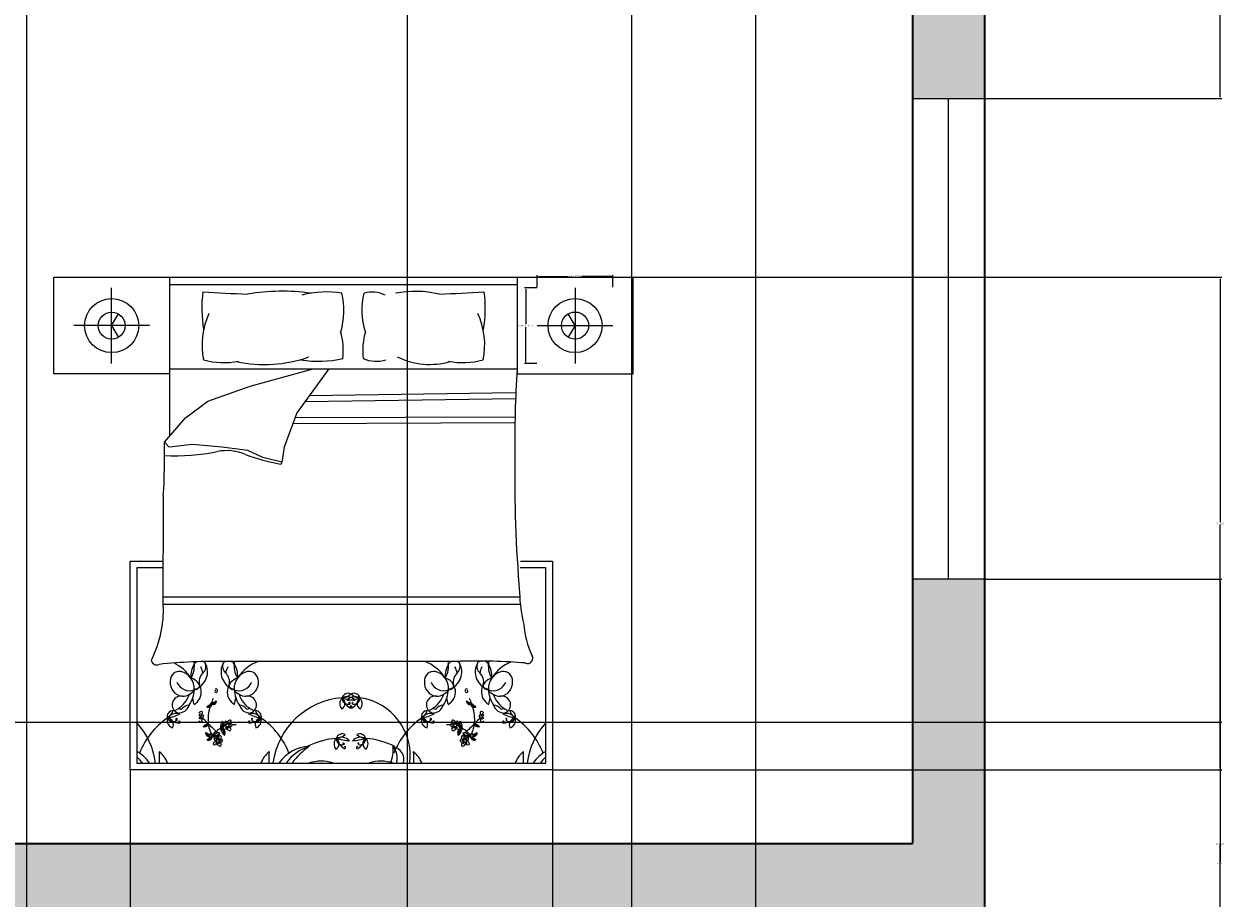
# Model space of a CAD drawing. Units: inches. Extents: x 0 to 423, y -517 to 94.
# Tile 5 of 8: x 273 to 423, y -270 to -160. Entities that reach past the tile are written whole.
import ezdxf

# ---------------------------------------------------------------- set-up
doc = ezdxf.new("R2010")
doc.units = ezdxf.units.IN
doc.header["$MEASUREMENT"] = 0
for name, color, linetype, lineweight in [('A-ANNO-DIMS', 2, 'Continuous', 18), ('A-FURN', 8, 'Continuous', 13), ('A-GLAZ', 4, 'Continuous', 18), ('A-WALL', 7, 'Continuous', 35)]:
    doc.layers.add(name, color=color, linetype=linetype, lineweight=lineweight)
doc.layers.add('A-WALL-PATT', color=30, linetype='Continuous', lineweight=13, true_color=0xf26722)
doc.styles.get("Standard").update_dxf_attribs({"font": 'arial.ttf'})
doc.dimstyles.get("Standard").update_dxf_attribs({"dimtxt": 0.18, "dimasz": 0.18, "dimexe": 0.18, "dimexo": 0.0625, "dimgap": 0.09, "dimtad": 0, "dimtih": 1, "dimtoh": 1, "dimdec": 0, "dimzin": 0, "dimdsep": 46, "dimlunit": 3, "dimtxsty": 'Standard', "dimcen": 0.09, "dimadec": 0, "dimazin": 0, "dimtfac": 1, "dimtdec": 0, "dimtofl": 0, "dimtmove": 0, "dimatfit": 3, "dimfxl": 1, "dimtolj": 1, "dimtzin": 0, "dimarcsym": 0})

# ---------------------------------------------------------------- blocks, each defined once
blk = doc.blocks.new('WIN-GLAZ-60IN')
for p, q in [((0, 60), (0, 0)), ((4.5, 60), (4.5, 0)), ((9, 0), (9, 60))]:
    blk.add_line(p, q)
blk = doc.blocks.new('BEDSIDE-LAMP-MEDIUM')
for p, q in [((4.72, 0), (4.72, 9.44)), ((9.44, 4.72), (0, 4.72))]:
    blk.add_line(p, q)
for points in [[(4.72, 4.72), (5.56, 6.18)], [(4.72, 4.72), (5.56, 3.26)]]:
    blk.add_lwpolyline(points)
for radius in [3.37, 1.69]:
    blk.add_circle((4.72, 4.72), radius)
blk = doc.blocks.new('*D26')
at = {"layer": 'A-ANNO-DIMS', "color": 0, "lineweight": -2, "transparency": 16777216}
for p, q in [((336.85, -193.39), (335.32, -193.39)), ((335.5, -193.57), (335.5, -197.93)), ((335.5, -202.66), (335.5, -198.3)), ((336.85, -202.84), (335.32, -202.84))]:
    blk.add_line(p, q, dxfattribs=at)
at = {"layer": 'A-ANNO-DIMS', "color": 0, "transparency": 16777216}
for points in [[(335.47, -193.57), (335.53, -193.57), (335.5, -193.39)], [(335.47, -202.66), (335.53, -202.66), (335.5, -202.84)]]:
    blk.add_solid(points, dxfattribs=at)
at = {"layer": 'Defpoints', "color": 0, "transparency": 16777216}
for p in [(336.91, -193.39), (335.5, -202.84), (336.91, -202.84)]:
    blk.add_point(p, dxfattribs=at)
at = {"layer": 'A-ANNO-DIMS', "color": 0, "transparency": 16777216, "insert": (335.5, -198.12), "char_height": 0.18, "attachment_point": 5}
blk.add_mtext('\\A1;LAMP 0\'-9 1/2" TYP.', dxfattribs=at)
blk = doc.blocks.new('*D27')
at = {"layer": 'A-ANNO-DIMS', "color": 0, "lineweight": -2, "transparency": 16777216}
for p, q in [((336.91, -193.33), (336.91, -191.8)), ((337.09, -191.98), (340.78, -191.98)), ((346.17, -191.98), (342.48, -191.98)), ((346.35, -193.33), (346.35, -191.8))]:
    blk.add_line(p, q, dxfattribs=at)
at = {"layer": 'A-ANNO-DIMS', "color": 0, "transparency": 16777216}
for points in [[(337.09, -191.95), (337.09, -192.01), (336.91, -191.98)], [(346.17, -191.95), (346.17, -192.01), (346.35, -191.98)]]:
    blk.add_solid(points, dxfattribs=at)
at = {"layer": 'Defpoints', "color": 0, "transparency": 16777216}
for p in [(336.91, -191.98), (336.91, -193.39), (346.35, -193.39)]:
    blk.add_point(p, dxfattribs=at)
at = {"layer": 'A-ANNO-DIMS', "color": 0, "transparency": 16777216, "insert": (341.63, -191.98), "char_height": 0.18, "attachment_point": 5}
blk.add_mtext('\\A1;0\'-9 1/2" TYP.', dxfattribs=at)
blk = doc.blocks.new('*D35')
at = {"layer": 'A-ANNO-DIMS', "color": 0, "lineweight": -2, "transparency": 16777216}
for p, q in [((320.72, -389.7), (320.72, 45.81)), ((320.9, 45.63), (334.39, 45.63)), ((348.54, 45.63), (335.05, 45.63)), ((348.72, -389.7), (348.72, 45.81))]:
    blk.add_line(p, q, dxfattribs=at)
at = {"layer": 'A-ANNO-DIMS', "color": 0, "transparency": 16777216}
for points in [[(320.9, 45.66), (320.9, 45.6), (320.72, 45.63)], [(348.54, 45.66), (348.54, 45.6), (348.72, 45.63)]]:
    blk.add_solid(points, dxfattribs=at)
at = {"layer": 'Defpoints', "color": 0, "transparency": 16777216}
for p in [(348.72, 45.63), (320.72, -389.77), (348.72, -389.77)]:
    blk.add_point(p, dxfattribs=at)
at = {"layer": 'A-ANNO-DIMS', "color": 0, "transparency": 16777216, "insert": (334.72, 45.63), "char_height": 0.18, "attachment_point": 5}
blk.add_mtext('\\A1;2\'-4"', dxfattribs=at)
blk = doc.blocks.new('*D43')
at = {"layer": 'A-ANNO-DIMS', "color": 0, "lineweight": -2, "transparency": 16777216}
for p, q in [((392.79, -91.27), (422.3, -91.27)), ((422.12, -91.45), (422.12, -130.33)), ((422.12, -169.59), (422.12, -130.7)), ((392.79, -169.77), (422.3, -169.77))]:
    blk.add_line(p, q, dxfattribs=at)
at = {"layer": 'A-ANNO-DIMS', "color": 0, "transparency": 16777216}
for points in [[(422.09, -91.45), (422.15, -91.45), (422.12, -91.27)], [(422.09, -169.59), (422.15, -169.59), (422.12, -169.77)]]:
    blk.add_solid(points, dxfattribs=at)
at = {"layer": 'Defpoints', "color": 0, "transparency": 16777216}
for p in [(392.72, -91.27), (392.72, -169.77), (422.12, -169.77)]:
    blk.add_point(p, dxfattribs=at)
at = {"layer": 'A-ANNO-DIMS', "color": 0, "transparency": 16777216, "insert": (422.12, -130.52), "char_height": 0.18, "attachment_point": 5}
blk.add_mtext('\\A1;6\'-6 1/2"', dxfattribs=at)
blk = doc.blocks.new('*D44')
at = {"layer": 'A-ANNO-DIMS', "color": 0, "lineweight": -2, "transparency": 16777216}
for p, q in [((392.79, -229.77), (422.3, -229.77)), ((422.12, -229.95), (422.12, -265.08)), ((422.12, -300.59), (422.12, -265.45)), ((392.79, -300.77), (422.3, -300.77))]:
    blk.add_line(p, q, dxfattribs=at)
at = {"layer": 'A-ANNO-DIMS', "color": 0, "transparency": 16777216}
for points in [[(422.09, -229.95), (422.15, -229.95), (422.12, -229.77)], [(422.09, -300.59), (422.15, -300.59), (422.12, -300.77)]]:
    blk.add_solid(points, dxfattribs=at)
at = {"layer": 'Defpoints', "color": 0, "transparency": 16777216}
for p in [(392.72, -229.77), (392.72, -300.77), (422.12, -300.77)]:
    blk.add_point(p, dxfattribs=at)
at = {"layer": 'A-ANNO-DIMS', "color": 0, "transparency": 16777216, "insert": (422.12, -265.27), "char_height": 0.18, "attachment_point": 5}
blk.add_mtext('\\A1;5\'-11"', dxfattribs=at)
blk = doc.blocks.new('*D50')
at = {"layer": 'A-ANNO-DIMS', "color": 0, "lineweight": -2, "transparency": 16777216}
for p, q in [((273.19, -103.61), (273.19, -517.35)), ((364.14, -103.61), (364.14, -517.35)), ((273.37, -517.17), (318.34, -517.17)), ((363.96, -517.17), (318.99, -517.17))]:
    blk.add_line(p, q, dxfattribs=at)
at = {"layer": 'A-ANNO-DIMS', "color": 0, "transparency": 16777216}
for points in [[(273.37, -517.14), (273.37, -517.2), (273.19, -517.17)], [(363.96, -517.14), (363.96, -517.2), (364.14, -517.17)]]:
    blk.add_solid(points, dxfattribs=at)
at = {"layer": 'Defpoints', "color": 0, "transparency": 16777216}
for p in [(273.19, -103.55), (364.14, -103.55), (364.14, -517.17)]:
    blk.add_point(p, dxfattribs=at)
at = {"layer": 'A-ANNO-DIMS', "color": 0, "transparency": 16777216, "insert": (318.66, -517.17), "char_height": 0.18, "attachment_point": 5}
blk.add_mtext('\\A1;7\'-7"', dxfattribs=at)
blk = doc.blocks.new('*D51')
at = {"layer": 'A-ANNO-DIMS', "color": 0, "lineweight": -2, "transparency": 16777216}
for p, q in [((286.14, -253.61), (286.14, -517.35)), ((338.82, -253.61), (338.82, -517.35)), ((286.32, -517.17), (311.93, -517.17)), ((338.64, -517.17), (313.02, -517.17))]:
    blk.add_line(p, q, dxfattribs=at)
at = {"layer": 'A-ANNO-DIMS', "color": 0, "transparency": 16777216}
for points in [[(286.32, -517.14), (286.32, -517.2), (286.14, -517.17)], [(338.64, -517.14), (338.64, -517.2), (338.82, -517.17)]]:
    blk.add_solid(points, dxfattribs=at)
at = {"layer": 'Defpoints', "color": 0, "transparency": 16777216}
for p in [(286.14, -253.55), (338.82, -253.55), (338.82, -517.17)]:
    blk.add_point(p, dxfattribs=at)
at = {"layer": 'A-ANNO-DIMS', "color": 0, "transparency": 16777216, "insert": (312.48, -517.17), "char_height": 0.18, "attachment_point": 5}
blk.add_mtext('\\A1;4\'-4 1/2"', dxfattribs=at)
blk = doc.blocks.new('*D53')
at = {"layer": 'A-ANNO-DIMS', "color": 0, "lineweight": -2, "transparency": 16777216}
for p, q in [((85.83, -247.61), (422.3, -247.61)), ((422.12, -247.79), (422.12, -262.66)), ((422.12, -277.89), (422.12, -263.02)), ((80.68, -278.07), (422.3, -278.07))]:
    blk.add_line(p, q, dxfattribs=at)
at = {"layer": 'A-ANNO-DIMS', "color": 0, "transparency": 16777216}
for points in [[(422.09, -247.79), (422.15, -247.79), (422.12, -247.61)], [(422.09, -277.89), (422.15, -277.89), (422.12, -278.07)]]:
    blk.add_solid(points, dxfattribs=at)
at = {"layer": 'Defpoints', "color": 0, "transparency": 16777216}
for p in [(85.77, -247.61), (80.61, -278.07), (422.12, -278.07)]:
    blk.add_point(p, dxfattribs=at)
at = {"layer": 'A-ANNO-DIMS', "color": 0, "transparency": 16777216, "insert": (422.12, -262.84), "char_height": 0.18, "attachment_point": 5}
blk.add_mtext('\\A1;2\'-6 1/2"', dxfattribs=at)
blk = doc.blocks.new('*D61')
at = {"layer": 'A-ANNO-DIMS', "color": 0, "lineweight": -2, "transparency": 16777216}
for p, q in [((348.92, -192.09), (422.3, -192.09)), ((422.12, -192.27), (422.12, -222.64)), ((422.12, -253.37), (422.12, -223)), ((338.88, -253.55), (422.3, -253.55))]:
    blk.add_line(p, q, dxfattribs=at)
at = {"layer": 'A-ANNO-DIMS', "color": 0, "transparency": 16777216}
for points in [[(422.09, -192.27), (422.15, -192.27), (422.12, -192.09)], [(422.09, -253.37), (422.15, -253.37), (422.12, -253.55)]]:
    blk.add_solid(points, dxfattribs=at)
at = {"layer": 'Defpoints', "color": 0, "transparency": 16777216}
for p in [(348.86, -192.09), (338.82, -253.55), (422.12, -253.55)]:
    blk.add_point(p, dxfattribs=at)
at = {"layer": 'A-ANNO-DIMS', "color": 0, "transparency": 16777216, "insert": (422.12, -222.82), "char_height": 0.18, "attachment_point": 5}
blk.add_mtext('\\A1;5\'-1 1/2"', dxfattribs=at)

msp = doc.modelspace()

# ---------------------------------------------------------------- hatches: boundary and pattern name
at = {"layer": 'A-WALL-PATT'}
h = msp.add_hatch(color=256, dxfattribs=at)
h.dxf.hatch_style = 1
h.paths.add_polyline_path([(201.52, 16.23), (138.22, 16.23), (138.22, 7.23), (177.72, 7.23), (177.72, -138.77), (186.72, -138.77), (186.72, -92.77), (251.72, -92.77), (251.72, -22.53), (242.72, -22.53), (242.72, -83.77), (186.72, -83.77), (186.72, 7.23), (201.52, 7.23)])
h.paths.add_polyline_path([(78.22, 16.23), (29.72, 16.23), (29.72, -31.27), (38.72, -31.27), (38.72, 7.23), (78.22, 7.23)])
h.paths.add_polyline_path([(275.31, 16.23), (225.52, 16.23), (225.52, 7.23), (275.31, 7.23)])
h.paths.add_polyline_path([(392.72, 16.23), (335.31, 16.23), (335.31, 7.23), (383.72, 7.23), (383.72, -31.27), (392.72, -31.27)])
h.paths.add_polyline_path([(143.33, -129.77), (38.72, -129.77), (38.72, -91.27), (29.72, -91.27), (29.72, -157.27), (38.72, -157.27), (38.72, -138.77), (143.33, -138.77)])
h.paths.add_polyline_path([(186.72, -199.77), (38.72, -199.77), (38.72, -181.27), (29.72, -181.27), (29.72, -239.27), (38.72, -239.27), (38.72, -208.77), (177.72, -208.77), (177.72, -237.07), (186.72, -237.07)])
h.paths.add_polyline_path([(111.72, -161.55), (102.72, -161.55), (102.72, -199.77), (111.72, -199.77)])
h.paths.add_polyline_path([(392.72, -91.27), (383.72, -91.27), (383.72, -129.77), (242.72, -129.77), (242.72, -138.77), (383.72, -138.77), (383.72, -169.77), (392.72, -169.77)])
h.paths.add_polyline_path([(392.72, -229.77), (383.72, -229.77), (383.72, -262.77), (251.72, -262.77), (251.72, -177.14), (242.72, -177.14), (242.72, -271.77), (383.72, -271.77), (383.72, -300.77), (392.72, -300.77)])
h.paths.add_polyline_path([(392.72, -360.77), (383.72, -360.77), (383.72, -389.77), (378.42, -389.77), (378.42, -398.77), (383.72, -398.77), (383.72, -458.77), (382.72, -458.77), (382.72, -467.77), (392.72, -467.77)])
h.paths.add_polyline_path([(364.92, -389.77), (348.72, -389.77), (348.72, -467.77), (358.72, -467.77), (358.72, -458.77), (357.72, -458.77), (357.72, -398.77), (364.92, -398.77)])
h.paths.add_polyline_path([(320.72, -389.77), (283.72, -389.77), (283.72, -398.77), (320.72, -398.77)])
h.paths.add_polyline_path([(223.72, -389.77), (186.72, -389.77), (186.72, -270.38), (177.72, -270.38), (177.72, -458.77), (138.22, -458.77), (138.22, -467.77), (186.72, -467.77), (186.72, -398.77), (223.72, -398.77)])
h.paths.add_polyline_path([(143.29, -329.77), (38.72, -329.77), (38.72, -299.27), (29.72, -299.27), (29.72, -338.77), (143.29, -338.77)])
h.paths.add_polyline_path([(38.72, -374.71), (29.72, -374.71), (29.72, -398.74), (38.72, -398.74)])
h.paths.add_polyline_path([(78.22, -458.77), (38.72, -458.77), (38.72, -434.74), (29.72, -434.74), (29.72, -467.77), (78.22, -467.77)])
h.paths.add_polyline_path([(279.99, -158.17), (326.6, -158.17), (326.6, -135.78), (279.99, -135.78)], flags=25)
h.paths.add_polyline_path([(355.56, -439.13), (387, -439.13), (387, -416.66), (355.56, -416.66)], flags=9)

# ---------------------------------------------------------------- linework, layer by layer
at = {"layer": 'A-FURN'}
for p, q in [((276.6, -192.09), (348.86, -192.09)), ((291.05, -192.09), (291.05, -211.93)), ((334.41, -193.02), (291.05, -193.02)), ((291.05, -203.51), (334.41, -203.51)), ((301.09, -205.66), (308.97, -203.51)), ((310.9, -203.51), (306.94, -209.02)), ((295.82, -207.56), (301.09, -205.66)), ((334.21, -206.51), (308.49, -206.88)), ((293.04, -209.61), (295.82, -207.56)), ((334.18, -207.26), (307.95, -207.63)), ((306.94, -209.02), (305.33, -213.27)), ((334.15, -209.53), (306.71, -209.64)), ((290.4, -212.68), (293.04, -209.61)), ((334.15, -210.27), (306.42, -210.39)), ((290.99, -213.27), (290.4, -212.68)), ((293.92, -212.97), (290.99, -213.27)), ((297.57, -213.27), (293.92, -212.97)), ((300.79, -213.71), (297.57, -213.27)), ((302.7, -214.58), (300.79, -213.71)), ((305.33, -213.27), (305.04, -215.17)), ((305.04, -215.17), (302.7, -214.58)), ((286.14, -227.52), (290.22, -227.52)), ((286.14, -253.55), (286.14, -227.52)), ((334.81, -227.52), (338.82, -227.52)), ((338.82, -227.52), (338.82, -253.55)), ((290.22, -228.35), (286.97, -228.35)), ((286.97, -228.35), (286.97, -252.71)), ((337.98, -228.35), (334.79, -228.35)), ((337.98, -252.71), (337.98, -228.35)), ((334.73, -232.02), (290.22, -232.02)), ((334.8, -232.92), (290.22, -232.92)), ((327.4, -240.02), (298.06, -240.02)), ((294.09, -245.38), (293.93, -244.57)), ((299.14, -245.38), (299.3, -244.57)), ((325.81, -245.38), (325.65, -244.57)), ((330.86, -245.38), (331.02, -244.57)), ((286.97, -252.71), (337.98, -252.71)), ((338.82, -253.55), (286.14, -253.55))]:
    msp.add_line(p, q, dxfattribs=at)
for points in [[(291.05, -204.14), (276.6, -204.14), (276.6, -192.09)], [(334.41, -192.09), (334.41, -204.14), (348.86, -204.14), (348.86, -192.09)]]:
    msp.add_lwpolyline(points, dxfattribs=at)
for points in [[(295.2, -193.89, 0.074897), (295.29, -198.61, -0.472817)], [(312.39, -198.88, 0.14099), (312.53, -194.06, 0.235245)], [(315.48, -198.88, -0.14099), (315.33, -194.06, -0.235245)], [(330.26, -193.89, -0.074897), (330.17, -198.61, 0.472817)], [(290.25, -219.3, 0.001242), (290.22, -233.01, -0.127202), (288.77, -239.84)], [(334.71, -231.45, 0.056112), (335.24, -235.43, 0.095341), (336.25, -239.26)]]:
    msp.add_lwpolyline(points, format="xyb", dxfattribs=at)
for centre in [(298.27, -248), (326.68, -248), (297.06, -249.94), (327.89, -249.94)]:
    msp.add_circle(centre, 0.184, dxfattribs=at)
for centre, radius, start, end in [((335.03, 493.79), 688.84, 266.68521, 267.14978), ((305.1, -220.04), 26.21, 82.2196, 99.497), ((310.64, -206.8), 12.88, 81.5249, 103.96), ((316.32, -197.5), 3.57, 63.3437, 106.1026), ((321.68, -206.54), 12.7, 76.3427, 101.1841), ((290.43, 493.79), 688.84, 272.85022, 273.31479), ((304.41, -200.51), 9.31, 155.1316, 191.7583), ((321.05, -200.51), 9.31, 348.2417, 24.8684), ((303.87, -201.29), 8.85, 354.0129, 15.8293), ((323.99, -201.29), 8.85, 164.1707, 185.9871), ((302.88, -186.17), 16.8, 258.0397, 289.2615), ((323.5, -193.76), 9.2, 243.8761, 286.1746), ((297.78, -193.05), 9.68, 255.1039, 281.0369), ((309.68, -189.83), 12.74, 259.8617, 283.6238), ((316.81, -198.74), 3.83, 245.0183, 288.5407), ((327.68, -193.05), 9.68, 258.9631, 284.8961), ((463.95, -212.34), 129.84, 176.1, 180.9282), ((224.15, -214.48), 66.28, 355.8294, 1.553), ((291.64, -187.09), 27.27, 267.4519, 281.3392), ((298.16, -219.6), 5.88, 66.2616, 101.3392), ((310.06, -187.86), 28.02, 250.1194, 259.3383), ((304.87, -215.23), 0.174, 268.8623, 19.7536), ((503.47, -217.06), 169.37, 179.1145, 184.8735), ((335.71, -239.63), 0.659, 246.5219, 33.8264), ((289.43, -239.8), 0.667, 183.98, 297.3412), ((297.2, -315.24), 75.22, 89.3433, 95.6887), ((289.15, -245.11), 5.47, 33.6671, 63.2997), ((296.48, -241.86), 2.79, 145.785, 184.7304), ((291.16, -240.56), 2.99, 328.8218, 9.1554), ((294.87, -240.82), 0.87, 120.0293, 142.325), ((293.48, -241.33), 2.3, 289.2822, 29.1751), ((293.13, -241.75), 2.08, 7.436, 29.9149), ((294.5, -240.65), 1.08, 311.5653, 23.8354), ((294.87, -240.82), 0.87, 44.4517, 63.558), ((299.76, -241.33), 2.3, 150.8249, 250.7178), ((298.74, -240.65), 1.08, 156.1646, 228.4347), ((298.37, -240.82), 0.87, 113.229, 135.5483), ((300.11, -241.75), 2.08, 150.0851, 172.564), ((298.37, -240.82), 0.87, 37.675, 66.7144), ((296.76, -241.86), 2.79, 355.2696, 34.215), ((302.08, -240.56), 2.99, 169.7133, 211.1782), ((304.09, -245.11), 5.47, 111.4941, 146.3329), ((320.87, -245.11), 5.47, 33.6671, 68.5059), ((328.2, -241.86), 2.79, 145.785, 184.7304), ((322.87, -240.56), 2.99, 328.8218, 10.2867), ((326.58, -240.82), 0.87, 113.2856, 142.325), ((325.19, -241.33), 2.3, 289.2822, 29.1751), ((324.84, -241.75), 2.08, 7.436, 29.9149), ((326.58, -240.82), 0.87, 44.4517, 66.7144), ((326.21, -240.65), 1.08, 311.5653, 23.8354), ((329.61, -310.3), 70.32, 85.2402, 91.8035), ((331.48, -241.33), 2.3, 150.8249, 250.7178), ((330.45, -240.65), 1.08, 156.1646, 228.4347), ((330.09, -240.82), 0.87, 106.6343, 135.5483), ((331.82, -241.75), 2.08, 150.0851, 172.564), ((330.09, -240.82), 0.87, 37.675, 72.5814), ((328.47, -241.86), 2.79, 355.2696, 34.215), ((333.79, -240.56), 2.99, 169.249, 211.1782), ((335.8, -245.11), 5.47, 113.6453, 146.3329), ((292.84, -242.66), 1.73, 174.9449, 262.8857), ((292.34, -242.48), 1.22, 84.4856, 181.0538), ((291.96, -243.39), 2.17, 355.2933, 76.921), ((293.2, -243.83), 1.8, 299.9085, 73.1337), ((296.2, -242.57), 1.48, 131.5653, 195.1471), ((297.04, -242.57), 1.48, 344.8529, 48.4347), ((300.04, -243.83), 1.8, 106.8663, 240.0915), ((301.27, -243.39), 2.17, 103.079, 184.7067), ((300.4, -242.66), 1.73, 277.1143, 5.0551), ((300.9, -242.48), 1.22, 358.9462, 95.5144), ((324.05, -242.48), 1.22, 84.4856, 181.0538), ((324.55, -242.66), 1.73, 174.9449, 262.8857), ((323.68, -243.39), 2.17, 355.2933, 76.921), ((324.91, -243.83), 1.8, 299.9085, 73.1337), ((327.91, -242.57), 1.48, 131.5653, 195.1471), ((328.75, -242.57), 1.48, 344.8529, 48.4347), ((331.75, -243.83), 1.8, 106.8663, 240.0915), ((332.99, -243.39), 2.17, 103.079, 184.7067), ((332.11, -242.66), 1.73, 277.1143, 5.0551), ((332.61, -242.48), 1.22, 358.9462, 95.5144), ((293.52, -242), 1.68, 201.5819, 291.4221), ((292.54, -242.28), 2.1, 272.3591, 324.0401), ((290.26, -243.33), 3.88, 326.2883, 356.5076), ((296.48, -241.86), 2.79, 212.7011, 216.3445), ((294.34, -243.07), 0.449, 257.3041, 15.1471), ((296.83, -243.75), 0.139, 102.7051, 280.4384), ((296.81, -243.67), 0.226, 280.4384, 100.4136), ((298.9, -243.07), 0.449, 164.8529, 282.6959), ((296.76, -241.86), 2.79, 323.6555, 327.2989), ((300.7, -242.28), 2.1, 215.9599, 267.6409), ((299.72, -242), 1.68, 248.5779, 338.4181), ((302.98, -243.33), 3.88, 183.4924, 213.7117), ((313.31, -244.79), 0.782, 63.0274, 163.8037), ((314.05, -244.79), 0.782, 16.1963, 116.9726), ((325.23, -242), 1.68, 201.5819, 291.4221), ((324.25, -242.28), 2.1, 272.3591, 324.0401), ((321.97, -243.33), 3.88, 326.2883, 356.5076), ((328.2, -241.86), 2.79, 212.7011, 216.3445), ((326.05, -243.07), 0.449, 257.3041, 15.1471), ((328.14, -243.67), 0.226, 79.5864, 259.5616), ((328.13, -243.75), 0.139, 259.5616, 77.2949), ((330.62, -243.07), 0.449, 164.8529, 282.6959), ((328.47, -241.86), 2.79, 323.6555, 327.2989), ((332.41, -242.28), 2.1, 215.9599, 267.6409), ((331.44, -242), 1.68, 248.5779, 338.4181), ((334.69, -243.33), 3.88, 183.4924, 213.7117), ((292.44, -245.44), 1.08, 80.264, 250.8688), ((290.29, -243.05), 3.41, 301.2614, 341.7045), ((292.18, -245.12), 1.35, 265.969, 344.3045), ((293.64, -246.92), 1.44, 96.1662, 141.5825), ((295.24, -244.62), 1.16, 308.2101, 316.3071), ((295.95, -245.38), 0.347, 278.3432, 4.2869), ((295.76, -245.08), 0.606, 300.656, 332.6341), ((296.21, -245.48), 0.147, 55.7657, 157.4417), ((301.83, -247.39), 5.99, 153.0032, 159.8941), ((296.44, -245.34), 0.147, 84.3784, 186.0543), ((296.3, -244.75), 0.606, 269.1859, 301.164), ((296.48, -245.06), 0.347, 237.5332, 323.4768), ((296.14, -244.08), 1.16, 285.5129, 293.6099), ((296.9, -245.38), 0.379, 87.3579, 140.4944), ((296.02, -244.29), 1.14, 301.164, 321.5612), ((295.1, -244.09), 2.04, 324.6898, 333.4936), ((302.95, -243.05), 3.41, 198.2955, 238.7386), ((299.6, -246.92), 1.44, 38.4175, 83.8338), ((301.06, -245.12), 1.35, 195.6955, 274.031), ((300.8, -245.44), 1.08, 289.1312, 99.736), ((313.29, -253.98), 9.44, 94.4623, 172.255), ((313.33, -245.28), 1.05, 137.7873, 219.1145), ((312.14, -245.24), 0.788, 298.5391, 58.3627), ((313.33, -244.6), 0.772, 177.7585, 283.852), ((312.51, -242.96), 1.61, 271.4585, 315.3727), ((313.17, -245.93), 1.49, 45.5411, 114.3101), ((314.53, -238.27), 6.6, 252.593, 267.2582), ((314.81, -243.8), 2.39, 198.9159, 238.011), ((314.19, -245.93), 1.49, 65.6899, 134.4589), ((312.83, -238.27), 6.6, 272.7418, 287.407), ((313.49, -245.25), 0.102, 283.852, 219.9245), ((314.85, -242.96), 1.61, 224.6273, 268.5415), ((313.86, -245.21), 0.0615, 320.1909, 256.0209), ((312.55, -243.8), 2.39, 301.989, 341.0841), ((314.03, -244.6), 0.772, 256.148, 2.2415), ((315.22, -245.24), 0.788, 121.6373, 241.4609), ((314.03, -245.28), 1.05, 320.8855, 42.2127), ((313.77, -251.8), 7.3, 352.8636, 81.8197), ((324.16, -245.44), 1.08, 80.264, 250.8688), ((322.01, -243.05), 3.41, 301.2614, 341.7045), ((323.89, -245.12), 1.35, 265.969, 344.3045), ((325.35, -246.92), 1.44, 96.1662, 141.5825), ((328.93, -244.29), 1.14, 218.4388, 238.836), ((328.05, -245.38), 0.379, 39.5056, 92.6421), ((329.86, -244.09), 2.04, 206.5064, 215.3102), ((328.47, -245.06), 0.347, 216.5232, 302.4668), ((328.81, -244.08), 1.16, 246.3901, 254.4871), ((328.65, -244.75), 0.606, 238.836, 270.8141), ((323.12, -247.39), 5.99, 20.1059, 26.9968), ((328.51, -245.34), 0.147, 353.9457, 95.6216), ((328.74, -245.48), 0.147, 22.5583, 124.2343), ((329, -245.38), 0.347, 175.7131, 261.6568), ((329.2, -245.08), 0.606, 207.3659, 239.344), ((329.72, -244.62), 1.16, 223.6929, 231.7899), ((334.66, -243.05), 3.41, 198.2955, 238.7386), ((332.77, -245.12), 1.35, 195.6955, 274.031), ((331.31, -246.92), 1.44, 38.4175, 83.8338), ((332.51, -245.44), 1.08, 289.1312, 99.736), ((291.52, -246.94), 0.782, 92.9516, 193.728), ((289.92, -245.75), 1.61, 301.3827, 345.2969), ((291.97, -248), 1.49, 75.4653, 144.2343), ((289.33, -240.68), 6.6, 282.5173, 297.1824), ((292.22, -246.62), 0.665, 63.9755, 143.2681), ((294.96, -246.62), 0.307, 101.5637, 142.6358), ((294.7, -246.91), 0.184, 273.2768, 86.7232), ((294.92, -246.73), 0.176, 91.1081, 181.8675), ((295.1, -247.09), 0.38, 80.3487, 133.6538), ((295.03, -246.77), 0.301, 229.7889, 317.6792), ((294.71, -246.38), 0.443, 288.7263, 352.5032), ((295.03, -247.48), 0.602, 83.0852, 105.7171), ((295.01, -246.4), 0.142, 345.2356, 144.9248), ((295.14, -246.87), 0.159, 317.6792, 80.3487), ((296.03, -245.9), 0.379, 101.3256, 154.4621), ((295.48, -244.62), 1.14, 280.2588, 300.656), ((295.75, -243.7), 2.04, 268.3264, 277.1302), ((301.83, -247.39), 5.99, 163.5842, 183.8277), ((301.02, -246.62), 0.665, 36.7319, 116.0245), ((301.26, -248), 1.49, 35.7657, 104.5347), ((303.91, -240.68), 6.6, 242.8176, 257.4827), ((301.72, -246.94), 0.782, 346.272, 87.0484), ((303.31, -245.75), 1.61, 194.7031, 238.6173), ((313.61, -245.72), 0.117, 238.011, 71.5592), ((313.63, -245.67), 0.0569, 71.5592, 188.0167), ((313.75, -245.72), 0.117, 108.4408, 301.989), ((313.73, -245.67), 0.0569, 351.9833, 108.4408), ((323.24, -246.94), 0.782, 92.9516, 193.728), ((321.64, -245.75), 1.61, 301.3827, 345.2969), ((323.69, -248), 1.49, 75.4653, 144.2343), ((321.05, -240.68), 6.6, 282.5173, 297.1824), ((323.93, -246.62), 0.665, 63.9755, 143.2681), ((323.12, -247.39), 5.99, 356.1723, 16.4158), ((329.47, -244.62), 1.14, 239.344, 259.7412), ((329.21, -243.7), 2.04, 262.8698, 271.6736), ((328.92, -245.9), 0.379, 25.5379, 78.6744), ((329.81, -246.87), 0.159, 99.6513, 222.3208), ((329.92, -246.77), 0.301, 222.3208, 310.2111), ((329.85, -247.09), 0.38, 46.3462, 99.6513), ((329.94, -246.4), 0.142, 35.0752, 194.7644), ((330.24, -246.38), 0.443, 187.4968, 251.2737), ((329.92, -247.48), 0.602, 74.2829, 96.9148), ((330.04, -246.73), 0.176, 358.1325, 88.8919), ((330, -246.62), 0.307, 37.3642, 78.4363), ((330.25, -246.91), 0.184, 93.2768, 266.7232), ((332.73, -246.62), 0.665, 36.7319, 116.0245), ((332.98, -248), 1.49, 35.7657, 104.5347), ((335.62, -240.68), 6.6, 242.8176, 257.4827), ((335.03, -245.75), 1.61, 194.7031, 238.6173), ((333.43, -246.94), 0.782, 346.272, 87.0484), ((279.95, -253.98), 9.44, 7.745, 41.8856), ((296.09, -254.91), 9.44, 124.3865, 158.5908), ((291.78, -247.35), 1.05, 167.7115, 249.0387), ((290.74, -247.91), 0.788, 328.4633, 88.2869), ((292.33, -245.33), 2.39, 228.8402, 267.9352), ((291.45, -246.77), 0.772, 207.6827, 313.7762), ((291.91, -247.25), 0.102, 313.7762, 249.7183), ((292.24, -247.54), 0.0569, 101.4834, 217.9409), ((292.25, -247.6), 0.117, 267.9352, 101.4834), ((294.95, -247.25), 0.304, 217.7621, 259.0403), ((295.28, -246.84), 0.559, 203.4276, 227.6104), ((294.69, -247.41), 0.428, 355.053, 68.3618), ((294.98, -247.44), 0.141, 232.4737, 355.053), ((290.86, -252.48), 6.86, 43.1541, 52.0459), ((295.6, -248.34), 0.379, 101.3256, 154.4621), ((295.05, -247.05), 1.14, 280.2588, 300.656), ((295.31, -246.13), 2.04, 268.3264, 277.1302), ((294.8, -247.05), 1.16, 308.2101, 316.3071), ((295.52, -247.81), 0.347, 278.3432, 4.2869), ((295.33, -247.51), 0.606, 300.656, 332.6341), ((295.78, -247.91), 0.147, 55.7657, 157.4417), ((298.85, -247.54), 3, 184.756, 209.2041), ((303.17, -241.15), 9.87, 222.2412, 232.1744), ((299.16, -251.52), 3.6, 120.544, 139.818), ((296.86, -247.73), 0.839, 304.5369, 16.3699), ((297.31, -247.92), 0.51, 272.8499, 356.1226), ((296.95, -248.11), 0.494, 321.7607, 7.9252), ((297.05, -248.82), 0.494, 8.7227, 54.8872), ((297.08, -249.22), 0.839, 0.278, 72.111), ((298.02, -247.96), 0.593, 127.3105, 187.9252), ((297.45, -248.91), 0.51, 20.5253, 88.5375), ((297.21, -247.9), 0.609, 355.0106, 41.658), ((297.88, -248.35), 0.182, 148.0499, 225.6268), ((299.16, -251.52), 3.6, 113.0501, 113.8477), ((298.22, -248.56), 0.58, 104.7558, 148.0499), ((297.89, -248.14), 0.363, 247.4086, 351.4386), ((298.07, -247.75), 0.251, 126.1046, 271.4281), ((298.04, -247.68), 0.18, 353.7526, 131.7054), ((298, -248.16), 0.122, 262.906, 7.132), ((297.87, -247.89), 0.253, 0.0645, 61.1507), ((297.93, -247.68), 0.289, 311.8413, 355.7877), ((298.52, -247.72), 0.307, 101.5637, 176.365), ((298.52, -248.34), 0.304, 151.2196, 259.0403), ((298.48, -247.83), 0.176, 91.1081, 181.8675), ((298.85, -247.94), 0.559, 203.4276, 227.6104), ((298.67, -248.18), 0.38, 80.3487, 133.6538), ((298.6, -247.87), 0.301, 229.7889, 317.6792), ((298.28, -247.48), 0.443, 288.7263, 352.5032), ((298.26, -248.5), 0.428, 355.053, 68.3618), ((298.6, -248.58), 0.602, 83.0852, 105.7171), ((298.58, -247.5), 0.142, 345.2356, 144.9248), ((298.71, -247.96), 0.159, 317.6792, 80.3487), ((299.16, -251.52), 3.6, 87.1071, 94.7585), ((300.99, -247.6), 0.117, 78.5166, 272.0648), ((300.9, -245.33), 2.39, 272.0648, 311.1598), ((301, -247.54), 0.0569, 322.0591, 78.5166), ((301.79, -246.77), 0.772, 226.2238, 332.3173), ((301.34, -247.21), 0.0615, 290.2667, 226.2271), ((302.5, -247.91), 0.788, 91.7131, 211.5367), ((301.45, -247.35), 1.05, 290.9613, 12.2885), ((297.15, -254.91), 9.44, 21.4092, 55.6135), ((327.81, -254.91), 9.44, 124.3865, 158.5908), ((323.5, -247.35), 1.05, 167.7115, 249.0387), ((323.16, -246.77), 0.772, 207.6827, 313.7762), ((324.05, -245.33), 2.39, 228.8402, 267.9352), ((322.45, -247.91), 0.788, 328.4633, 88.2869), ((323.62, -247.25), 0.102, 313.7762, 249.7183), ((323.95, -247.54), 0.0569, 101.4834, 217.9409), ((323.97, -247.6), 0.117, 267.9352, 101.4834), ((325.79, -251.52), 3.6, 85.2415, 92.8929), ((326.25, -247.96), 0.159, 99.6513, 222.3208), ((326.35, -247.87), 0.301, 222.3208, 310.2111), ((326.28, -248.18), 0.38, 46.3462, 99.6513), ((326.37, -247.5), 0.142, 35.0752, 194.7644), ((326.68, -247.48), 0.443, 187.4968, 251.2737), ((326.69, -248.5), 0.428, 111.6382, 184.947), ((326.35, -248.58), 0.602, 74.2829, 96.9148), ((326.47, -247.83), 0.176, 358.1325, 88.8919), ((326.1, -247.94), 0.559, 312.3896, 336.5724), ((326.43, -247.72), 0.307, 3.635, 78.4363), ((326.43, -248.34), 0.304, 280.9597, 28.7804), ((327.06, -248.14), 0.363, 188.5614, 292.5914), ((326.91, -247.68), 0.18, 48.2946, 186.2474), ((327.02, -247.68), 0.289, 184.2123, 228.1587), ((327.08, -247.89), 0.253, 118.8493, 179.9355), ((326.96, -248.16), 0.122, 172.868, 277.094), ((326.89, -247.75), 0.251, 268.5719, 53.8954), ((326.73, -248.56), 0.58, 31.9501, 75.2442), ((327.5, -248.91), 0.51, 91.4625, 159.4747), ((327.87, -249.22), 0.839, 107.889, 179.722), ((327.74, -247.9), 0.609, 138.342, 184.9894), ((327.64, -247.92), 0.51, 183.8774, 267.1501), ((325.79, -251.52), 3.6, 66.1523, 66.9499), ((327.07, -248.35), 0.182, 314.3732, 31.9501), ((328.09, -247.73), 0.839, 163.6301, 235.4631), ((326.93, -247.96), 0.593, 352.0748, 52.6895), ((327.9, -248.82), 0.494, 125.1128, 171.2773), ((328, -248.11), 0.494, 172.0748, 218.2393), ((325.79, -251.52), 3.6, 40.182, 59.456), ((321.78, -241.15), 9.87, 307.8256, 317.7588), ((326.1, -247.54), 3, 330.7959, 355.244), ((334.09, -252.48), 6.86, 127.9541, 136.8459), ((329.17, -247.91), 0.147, 22.5583, 124.2343), ((329.43, -247.81), 0.347, 175.7131, 261.6568), ((329.63, -247.51), 0.606, 207.3659, 239.344), ((330.15, -247.05), 1.16, 223.6929, 231.7899), ((329.9, -247.05), 1.14, 239.344, 259.7412), ((329.64, -246.13), 2.04, 262.8698, 271.6736), ((329.35, -248.34), 0.379, 25.5379, 78.6744), ((330.26, -247.41), 0.428, 111.6382, 184.947), ((329.97, -247.44), 0.141, 184.947, 307.5263), ((329.67, -246.84), 0.559, 312.3896, 336.5724), ((330, -247.25), 0.304, 280.9597, 322.2379), ((332.7, -247.6), 0.117, 78.5166, 272.0648), ((332.62, -245.33), 2.39, 272.0648, 311.1598), ((332.71, -247.54), 0.0569, 322.0591, 78.5166), ((333.51, -246.77), 0.772, 226.2238, 332.3173), ((333.05, -247.21), 0.0615, 290.2667, 226.2271), ((334.21, -247.91), 0.788, 91.7131, 211.5367), ((333.17, -247.35), 1.05, 290.9613, 12.2885), ((328.86, -254.91), 9.44, 21.4092, 55.6135), ((345, -253.98), 9.44, 138.1144, 172.255), ((295.73, -249), 0.205, 146.8636, 236.9021), ((298.62, -244.47), 5.38, 235.1882, 238.8844), ((296.08, -248.7), 0.556, 199.4799, 267.6828), ((296.02, -248.91), 0.479, 212.8155, 277.3992), ((295.74, -249.23), 0.556, 266.9701, 338.2913), ((292.81, -245.26), 5.38, 302.6784, 306.3746), ((295.88, -249.67), 0.205, 214.3538, 304.3923), ((295.95, -248.9), 0.213, 238.8844, 314.2646), ((295.91, -249.37), 0.479, 280.3057, 17.1958), ((295.87, -249.42), 0.213, 306.3746, 21.7548), ((296.21, -249.28), 0.161, 19.3605, 201.7548), ((296.21, -249.16), 0.161, 311.8703, 134.2646), ((299.23, -250.62), 3.21, 153.7819, 158.2913), ((296.68, -248.44), 0.839, 247.2305, 319.0635), ((296.4, -248.72), 0.494, 264.4544, 310.6188), ((298.85, -247.54), 3, 214.0033, 222.4917), ((296.77, -248.91), 0.51, 218.3208, 298.8162), ((297.02, -250.5), 0.58, 104.7558, 148.0499), ((296.86, -249.69), 0.251, 126.1046, 271.4281), ((296.83, -249.62), 0.18, 353.7526, 131.7054), ((297.11, -249.54), 0.593, 70.0041, 130.6188), ((296.66, -249.83), 0.253, 0.0645, 61.1507), ((296.72, -249.62), 0.289, 311.8413, 355.7877), ((296.73, -248.82), 0.609, 297.7043, 344.3516), ((297.32, -249.66), 0.307, 101.5637, 176.365), ((297.28, -249.77), 0.176, 91.1081, 181.8675), ((297.47, -250.12), 0.38, 80.3487, 133.6538), ((297.07, -249.42), 0.443, 288.7263, 352.5032), ((297.39, -250.52), 0.602, 83.0852, 105.7171), ((297.37, -249.44), 0.142, 345.2356, 144.9248), ((297.5, -249.9), 0.159, 317.6792, 80.3487), ((298.13, -248.66), 0.593, 188.7227, 249.3375), ((297.36, -248.96), 0.609, 334.9899, 21.6373), ((298.55, -248.53), 0.141, 232.4737, 355.053), ((312.57, -259.04), 9.44, 94.4623, 117.4146), ((312.61, -250.33), 1.05, 137.7873, 219.1145), ((311.42, -250.3), 0.788, 298.5391, 58.3627), ((312.58, -249.85), 0.782, 63.0274, 163.8037), ((311.79, -248.02), 1.61, 271.4585, 315.3727), ((312.45, -250.99), 1.49, 45.5411, 114.3101), ((314.09, -248.85), 2.39, 198.9159, 238.011), ((313.81, -243.33), 6.6, 252.593, 267.2582), ((312.6, -249.66), 0.772, 177.7585, 283.852), ((314.91, -250.99), 1.49, 65.6899, 134.4589), ((313.55, -243.33), 6.6, 272.7418, 287.407), ((314.78, -249.85), 0.782, 16.1963, 116.9726), ((315.57, -248.02), 1.61, 224.6273, 268.5415), ((313.27, -248.85), 2.39, 301.989, 341.0841), ((314.76, -249.66), 0.772, 256.148, 2.2415), ((315.94, -250.3), 0.788, 121.6373, 241.4609), ((314.75, -250.33), 1.05, 320.8855, 42.2127), ((314.79, -259.04), 9.44, 62.5854, 85.5377), ((326.4, -248.53), 0.141, 184.947, 307.5263), ((327.59, -248.96), 0.609, 158.3627, 205.0101), ((326.83, -248.66), 0.593, 290.6625, 351.2773), ((327.45, -249.9), 0.159, 99.6513, 222.3208), ((327.49, -250.12), 0.38, 46.3462, 99.6513), ((327.58, -249.44), 0.142, 35.0752, 194.7644), ((327.88, -249.42), 0.443, 187.4968, 251.2737), ((327.56, -250.52), 0.602, 74.2829, 96.9148), ((327.84, -249.54), 0.593, 49.3812, 109.9959), ((328.27, -248.44), 0.839, 220.9365, 292.7695), ((328.22, -248.82), 0.609, 195.6484, 242.2957), ((327.67, -249.77), 0.176, 358.1325, 88.8919), ((327.63, -249.66), 0.307, 3.635, 78.4363), ((328.19, -248.91), 0.51, 241.1838, 321.6792), ((328.12, -249.62), 0.18, 48.2946, 186.2474), ((328.23, -249.62), 0.289, 184.2123, 228.1587), ((328.29, -249.83), 0.253, 118.8493, 179.9355), ((328.09, -249.69), 0.251, 268.5719, 53.8954), ((327.94, -250.5), 0.58, 31.9501, 75.2442), ((328.55, -248.72), 0.494, 229.3812, 275.5456), ((326.1, -247.54), 3, 317.5083, 325.9967), ((329.04, -249.37), 0.479, 162.8042, 259.6943), ((328.74, -249.16), 0.161, 45.7354, 228.1297), ((328.74, -249.28), 0.161, 338.2452, 160.6395), ((325.72, -250.62), 3.21, 21.7087, 26.2181), ((329.21, -249.23), 0.556, 201.7087, 273.0299), ((329, -248.9), 0.213, 225.7354, 301.1156), ((328.94, -248.91), 0.479, 262.6008, 327.1845), ((329.08, -249.42), 0.213, 158.2452, 233.6254), ((328.87, -248.7), 0.556, 272.3172, 340.5201), ((332.15, -245.26), 5.38, 233.6254, 237.3216), ((329.07, -249.67), 0.205, 235.6077, 325.6462), ((326.33, -244.47), 5.38, 301.1156, 304.8118), ((329.23, -249), 0.205, 303.0979, 33.1364), ((284.68, -255.24), 4.6, 33.4617, 60.1116), ((287.26, -254.18), 3.84, 22.5547, 48.9546), ((276.75, -252.12), 13.06, 357.4081, 3.6519), ((296.68, -250.29), 0.182, 148.0499, 225.6268), ((296.69, -250.08), 0.363, 247.4086, 351.4386), ((296.79, -250.1), 0.122, 262.906, 7.132), ((297.32, -250.28), 0.304, 151.2196, 259.0403), ((297.64, -249.88), 0.559, 203.4276, 227.6104), ((297.4, -249.81), 0.301, 229.7889, 317.6792), ((297.06, -250.44), 0.428, 355.053, 68.3618), ((297.34, -250.47), 0.141, 232.4737, 355.053), ((305.98, -254.18), 3.84, 131.0454, 157.4453), ((316.49, -252.12), 13.06, 176.3481, 182.5919), ((308.56, -255.24), 4.6, 91.272, 146.5383), ((310.21, -256.1), 5.73, 107.8504, 143.6964), ((313.22, -257.71), 8.52, 124.0123, 144.053), ((312.76, -250.31), 0.102, 283.852, 219.9245), ((312.89, -250.78), 0.117, 238.011, 71.5592), ((312.91, -250.72), 0.0569, 71.5592, 188.0167), ((314.47, -250.78), 0.117, 108.4408, 301.989), ((314.45, -250.72), 0.0569, 351.9833, 108.4408), ((314.59, -250.27), 0.0615, 320.1909, 256.0209), ((314.71, -251.13), 4.22, 338.117, 6.6195), ((318.59, -252.31), 1.69, 346.3898, 79.0739), ((317.31, -252.08), 2.14, 342.8609, 41.9049), ((308.46, -252.12), 13.06, 357.4081, 3.6519), ((318.97, -254.18), 3.84, 22.5547, 48.9546), ((327.55, -249.81), 0.301, 222.3208, 310.2111), ((327.89, -250.44), 0.428, 111.6382, 184.947), ((327.61, -250.47), 0.141, 184.947, 307.5263), ((327.31, -249.88), 0.559, 312.3896, 336.5724), ((327.64, -250.28), 0.304, 280.9597, 28.7804), ((328.26, -250.08), 0.363, 188.5614, 292.5914), ((328.16, -250.1), 0.122, 172.868, 277.094), ((328.27, -250.29), 0.182, 314.3732, 31.9501), ((337.7, -254.18), 3.84, 131.0454, 157.4453), ((348.2, -252.12), 13.06, 176.3481, 182.5919), ((340.27, -255.24), 4.6, 119.8884, 146.5383), ((283.03, -256.1), 5.73, 36.3036, 46.4814), ((309.93, -257.67), 5.19, 73.5431, 107.0202), ((311.98, -260.34), 7.67, 94.3787, 95.6357), ((316.03, -265.6), 13.71, 109.7217, 109.9028), ((317.43, -257.67), 5.19, 72.9798, 106.4569), ((315.38, -260.34), 7.67, 84.3643, 85.6213), ((311.34, -265.6), 13.71, 70.0972, 70.2783), ((341.92, -256.1), 5.73, 133.5186, 143.6964)]:
    msp.add_arc(centre, radius, start, end, dxfattribs=at)
at = {"layer": 'A-GLAZ'}
for p, q in [((383.72, -169.77), (392.72, -169.77)), ((392.72, -229.77), (383.72, -229.77))]:
    msp.add_line(p, q, dxfattribs=at)
at = {"layer": 'A-WALL'}
for p, q in [((392.72, 16.23), (392.72, -467.77)), ((383.72, -138.77), (383.72, -199.77)), ((383.72, -199.77), (383.72, -208.77)), ((383.72, -208.77), (383.72, -262.77)), ((251.72, -262.77), (383.72, -262.77))]:
    msp.add_line(p, q, dxfattribs=at)

# ---------------------------------------------------------------- block references
at = {"layer": 'A-FURN'}
msp.add_blockref('BEDSIDE-LAMP-MEDIUM', (279.1, -202.84), dxfattribs=at)
at = {"layer": 'A-FURN', "rotation": 180}
msp.add_blockref('BEDSIDE-LAMP-MEDIUM', (346.35, -193.39), dxfattribs=at)
at = {"layer": 'A-GLAZ', "rotation": 180}
msp.add_blockref('WIN-GLAZ-60IN', (392.72, -169.77), dxfattribs=at)

# ---------------------------------------------------------------- dimensions: what is measured, and where the dimension line sits
at = {"layer": 'A-ANNO-DIMS'}
for base, p1, p2, picture, middle in [((348.72, 45.63), (320.72, -389.77), (348.72, -389.77), '*D35', (334.72, 45.63)), ((364.1422, -517.1651), (273.186, -103.5478), (364.1422, -103.5478), '*D50', (318.6641, -517.1651)), ((338.82, -517.17), (286.14, -253.55), (338.82, -253.55), '*D51', (312.48, -517.17))]:
    dim = msp.add_linear_dim(base=base, p1=p1, p2=p2, dimstyle='Standard', override={"dimdec": 1, "dimlfac": 1, "dimrnd": 0, "dimzin": 1, "dimdsep": 46, "dimlunit": 4, "dimfrac": 2}, dxfattribs=at)
    dim.commit()
    dim.dimension.update_dxf_attribs({"geometry": picture, "text_midpoint": middle})
for base, p1, p2, angle, picture, middle in [((422.12, -169.77), (392.72, -91.27), (392.72, -169.77), 270, '*D43', (422.12, -130.52)), ((422.12, -253.55), (348.86, -192.09), (338.82, -253.55), 90, '*D61', (422.12, -222.82)), ((422.12, -300.77), (392.72, -229.77), (392.72, -300.77), 270, '*D44', (422.12, -265.27)), ((422.12, -278.07), (85.77, -247.61), (80.61, -278.07), 90, '*D53', (422.12, -262.84))]:
    dim = msp.add_linear_dim(base=base, p1=p1, p2=p2, angle=angle, dimstyle='Standard', override={"dimdec": 1, "dimlfac": 1, "dimrnd": 0, "dimzin": 1, "dimdsep": 46, "dimlunit": 4, "dimfrac": 2}, dxfattribs=at)
    dim.commit()
    dim.dimension.update_dxf_attribs({"geometry": picture, "text_midpoint": middle})
for base, p1, p2, angle, text, picture, middle in [((336.91, -191.98), (346.35, -193.39), (336.91, -193.39), 180, '<> TYP.', '*D27', (341.63, -191.98)), ((335.4951, -202.8361), (336.9114, -193.394), (336.9114, -202.8361), 270, 'LAMP <> TYP.', '*D26', (335.4951, -198.1151))]:
    dim = msp.add_linear_dim(base=base, p1=p1, p2=p2, angle=angle, text=text, dimstyle='Standard', override={"dimdec": 1, "dimlfac": 1, "dimrnd": 0, "dimzin": 1, "dimdsep": 46, "dimlunit": 4, "dimfrac": 2}, dxfattribs=at)
    dim.commit()
    dim.dimension.update_dxf_attribs({"geometry": picture, "text_midpoint": middle})

doc.saveas('drawing.dxf')
